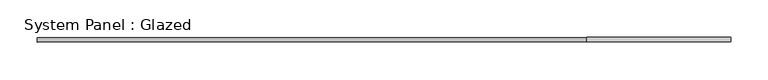
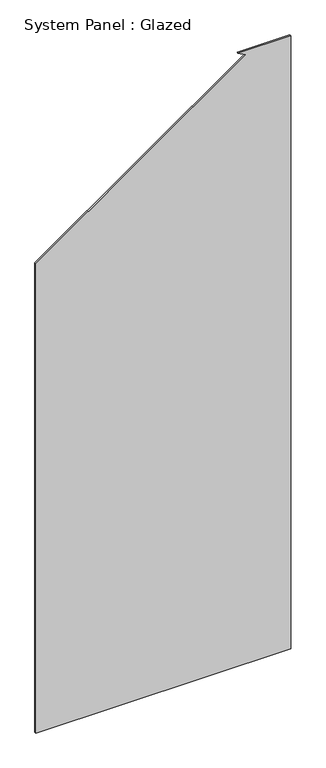
"""IFC4 building model written with IfcOpenShell, lengths in millimetres: plate geometry, System Panel : Glazed."""

from ifc_helpers import new_model, si_unit, frame, origin, place, context, project, spatial, polyline, outline, extrude, source, transform, mapped, element, save


def system_panel_glazed_60d66236(model_context):
    return source(origin(), model_context, "Body", "SweptSolid", [
        extrude(outline(polyline([(0.0, -462.5), (0.0, 462.5), (2350.0, 462.5), (2350.0, 270.5900419), (2334.0423978, 299.2688637), (1800.6460971, -462.5), (0.0, -462.5)])), frame((0.0, 34.0, 0.0), z_axis=(0.0, 1.0, 0.0), x_axis=(0.0, 0.0, 1.0)), (0.0, 0.0, 1.0), 6.0),
    ])


if __name__ == "__main__":
    model = new_model("IFC4")
    model_context = context("Model", 3, world=origin())
    ifc_project = project(units=[si_unit("LENGTHUNIT", "METRE", prefix="MILLI")], contexts=[model_context])
    site = spatial("IfcSite", under=ifc_project)
    building = spatial("IfcBuilding", under=site)
    placement = place(None, origin())
    system_panel_glazed_shape = system_panel_glazed_60d66236(model_context)
    element("IfcPlate", 1, ObjectType="System Panel : Glazed", at=placement, inside=building, context=model_context, shape_type="MappedRepresentation", body=[
        mapped(system_panel_glazed_shape, transform((0.0, 0.0, 0.0), x_axis=(1.0, 0.0, 0.0), y_axis=(0.0, 1.0, 0.0), z_axis=(0.0, 0.0, 1.0))),
    ])
    save(model, "model.ifc")

# Revit data of these elements
# Type "System Panel : Glazed"
#   Construction Type Id = "GSP4R"
#   Analytic Construction = "1/8 in Pilkington single glazing"
#   Visual Light Transmittance = 0.9
#   Solar Heat Gain Coefficient = 0.86
#   Heat Transfer Coefficient (U) = 6.7069 W/(m²·K)
#   Define Thermal Properties by = 1
# Element 1 (IfcPlate, "System Panel : Glazed")
#   Materials on its faces: "Default New Material(6)"
# Materials
#   "Default New Material(6)": class "Generic", colour RGB 191 25 25, transparency 0.9, Cost = 0
